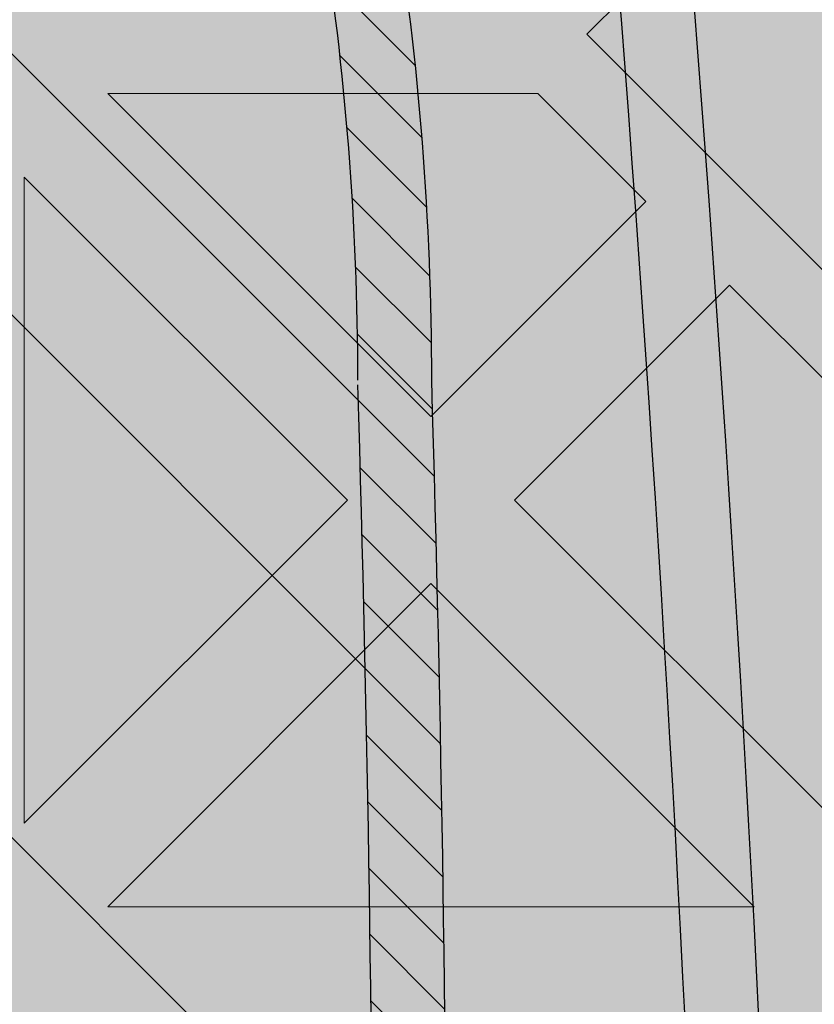
# Model space of a CAD drawing. Units: inches. Extents: x 844 to 2234, y 346 to 1084.
# Tile 38 of 93: x 1260.074 to 1261.788, y 699.229 to 701.353. Entities that reach past the tile are written whole.
import ezdxf

# ---------------------------------------------------------------- set-up
doc = ezdxf.new("R2010")
doc.units = ezdxf.units.IN
doc.header["$MEASUREMENT"] = 0
doc.layers.add('furniture', color=8, linetype='Continuous', lineweight=18)
doc.layers.add('RA-AP-01$0$INT', color=35, linetype='Continuous', lineweight=5)
doc.layers.add('RA-AP-01$0$FURN', color=3, linetype='Continuous')
doc.layers.add('RA-AP-01$0$WOOD', color=64, linetype='Continuous')

# ---------------------------------------------------------------- blocks, each defined once
blk = doc.blocks.new('A$C18D01794')
at = {"layer": 'RA-AP-01$0$INT'}
h = blk.add_hatch(color=256, dxfattribs=at)
h.paths.add_polyline_path([(4.585917135068448, -7.856712009587804), (4.614201406330596, -7.856712009587056), (4.668846067270487, -7.802067348644738), (4.723490728212344, -7.856712009584164), (4.771774999457151, -7.856712009582887), (4.826419660396886, -7.80206734864072), (4.862780050090322, -7.838427738332541), (4.844495778842715, -7.856712009580965), (4.862780050090411, -7.856712009580482), (4.905206456960182, -7.814285602707865), (4.947632863832445, -7.856712009578238), (4.965917135079675, -7.856712009577755), (4.947632863831759, -7.838427738330656), (4.983993253523576, -7.802067348637219), (5.038637914464627, -7.856712009575829), (5.08692218571208, -7.856712009574554), (5.141566846649976, -7.802067348634224), (5.196211507589851, -7.856712009571666), (5.224495778822615, -7.856712009570916), (4.905206456953975, -7.537422687702283)])
h.paths.add_polyline_path([(4.895206456956031, -7.575706958950402), (4.895206456958921, -7.684996280828174), (4.840561796018589, -7.630351619890275)], flags=16)
h.paths.add_polyline_path([(4.915206456955638, -7.575706958949956), (4.969851117895509, -7.630351619887399), (4.915206456957609, -7.684996280827732)], flags=16)
h.paths.add_polyline_path([(4.826419660395175, -7.644493755514321), (4.881064321335613, -7.699138416452331), (4.771774999456703, -7.69913841645522)], flags=16)
h.paths.add_polyline_path([(4.983993253519558, -7.644493755510815), (5.038637914460456, -7.699138416449285), (4.929348592581548, -7.69913841645126)], flags=16)
h.paths.add_polyline_path([(4.881064321336025, -7.719138416452334), (4.826419660397532, -7.773783077393256), (4.771774999457062, -7.719138416455217)], flags=16)
h.paths.add_polyline_path([(4.929348592582019, -7.71913841645126), (5.038637914460982, -7.719138416449284), (4.983993253522945, -7.773783077389749)], flags=16)
h.paths.add_polyline_path([(4.895206456960191, -7.733280552075633), (4.895206456962115, -7.806001331460164), (4.876922185715016, -7.824285602708492), (4.840561796021581, -7.787925213016675)], flags=16)
h.paths.add_polyline_path([(4.915206456958487, -7.733280552075187), (4.969851117899527, -7.787925213013798), (4.933490728206909, -7.824285602708034), (4.9152064569598, -7.806001331461736)], flags=16)
h.paths.add_polyline_path([(4.757632863832376, -7.733280552079264), (4.812277524772842, -7.787925213017304), (4.757632863834348, -7.842569873958233)], flags=16)
h.paths.add_polyline_path([(4.737632863832376, -7.73328055207979), (4.737632863834348, -7.842569873958701), (4.682988202893906, -7.787925213020692)], flags=16)
h.paths.add_polyline_path([(5.05278005008503, -7.733280552072701), (5.052780050087917, -7.842569873951664), (4.998135389146995, -7.787925213013169)], flags=16)
h.paths.add_polyline_path([(5.072780050085024, -7.733280552072333), (5.127424711025931, -7.787925213010806), (5.072780050087916, -7.842569873951244)], flags=16)
h.paths.add_polyline_path([(4.935917135072783, -7.506712009583784), (5.255206456948811, -7.826001331459767), (5.255206456948932, -7.797717060211899), (5.200561796010279, -7.743072399273238), (5.255206456949403, -7.688427738334128), (5.25520645694961, -7.640143467086677), (5.200561796009787, -7.585498806146837), (5.236922185702417, -7.549138416454212), (5.255206456949919, -7.56742268770172), (5.255206456949998, -7.549138416454178), (5.212780050078687, -7.506712009583814), (5.25520645695036, -7.464285602712145), (5.255206456950438, -7.446001331464763), (5.236922185702424, -7.464285602712779), (5.200561796009796, -7.427925213020149), (5.255206456950753, -7.373280552079203), (5.25520645695096, -7.324996280834394), (5.200561796010322, -7.270351619893748), (5.255206456951428, -7.215706958952649), (5.255206456951547, -7.187422687705071)])
h.paths.add_polyline_path([(5.042988202883395, -7.42792521302065), (5.097632863823085, -7.373280552080975), (5.097632863822622, -7.482569873959883)], flags=16)
h.paths.add_polyline_path([(5.028846067259663, -7.442067348644384), (5.083490728198774, -7.496712009583504), (4.974201406321001, -7.496712009583035)], flags=16)
h.paths.add_polyline_path([(5.117632863823087, -7.37328055208089), (5.172277524762331, -7.42792521302015), (5.11763286382262, -7.482569873959851)], flags=16)
h.paths.add_polyline_path([(5.08349072819877, -7.516712009582191), (5.028846067259652, -7.571356670521302), (4.974201406320998, -7.516712009582638)], flags=16)
h.paths.add_polyline_path([(5.131774999446817, -7.35913841645716), (5.186419660386065, -7.413783077396415), (5.241064321325782, -7.359138416456712)], flags=17)
h.paths.add_polyline_path([(5.131774999446228, -7.496712009583703), (5.186419660386065, -7.442067348643883), (5.222780050079488, -7.478427738337313), (5.204495778832781, -7.496712009584014)], flags=16)
h.paths.add_polyline_path([(5.097632863822613, -7.530854145205813), (5.097632863823061, -7.640143467084723), (5.042988202883383, -7.585498806145032)], flags=16)
h.paths.add_polyline_path([(5.131774999446899, -7.339138416457162), (5.241064321325809, -7.339138416456712), (5.186419660386591, -7.284493755517479)], flags=17)
h.paths.add_polyline_path([(5.131774999446226, -7.516712009581999), (5.204495778830767, -7.516712009581702), (5.22278005007868, -7.534996280829206), (5.186419660386049, -7.571356670521828)], flags=16)
h.paths.add_polyline_path([(5.11763286382262, -7.530854145205852), (5.17227752476232, -7.585498806145562), (5.117632863823064, -7.64014346708481)], flags=16)
h.paths.add_polyline_path([(5.186419660386069, -7.599640941770585), (5.241064321325754, -7.654285602710281), (5.131774999446791, -7.654285602709814)], flags=16)
h.paths.add_polyline_path([(5.131774999446872, -7.674285602709813), (5.24106432132578, -7.674285602710282), (5.186419660386554, -7.728930263649504)], flags=16)
h.paths.add_polyline_path([(5.255206456951811, -7.126001331467467), (5.255206456951895, -7.106712009588038), (4.555206456956052, -7.106712009588038), (4.555206456956136, -7.12600133146746), (4.905206456953973, -7.476001331465289)])
h.paths.add_polyline_path([(4.983993253513404, -7.368930263651977), (4.92934859257295, -7.314285602713969), (5.03863791445186, -7.314285602711063)], flags=16)
h.paths.add_polyline_path([(4.969851117889988, -7.383072399276016), (4.915206456952556, -7.437717060215906), (4.915206456949648, -7.328427738338133)], flags=16)
h.paths.add_polyline_path([(4.929348592572535, -7.294285602713971), (4.983993253511019, -7.239640941773039), (5.038637914451496, -7.294285602711065)], flags=16)
h.paths.add_polyline_path([(5.052780050074912, -7.280143467087016), (4.998135389134438, -7.225498806148989), (5.052780050072919, -7.170854145208052)], flags=16)
h.paths.add_polyline_path([(5.07278005007491, -7.280143467086489), (5.072780050072918, -7.170854145207579), (5.127424711013374, -7.225498806145578)], flags=16)
h.paths.add_polyline_path([(4.89520645695295, -7.437717060216355), (4.840561796013067, -7.383072399278919), (4.895206456950961, -7.328427738338582)], flags=16)
h.paths.add_polyline_path([(4.915206456948365, -7.280143467090674), (4.915206456946434, -7.207422687704125), (4.933490728192729, -7.18913841645701), (4.969851117886972, -7.225498806149623)], flags=16)
h.paths.add_polyline_path([(4.881064321327021, -7.314285602715054), (4.82641966038902, -7.368930263655506), (4.771774999448108, -7.314285602717047)], flags=16)
h.paths.add_polyline_path([(4.895206456950073, -7.280143467091125), (4.840561796009022, -7.225498806152518), (4.876922185700835, -7.18913841645908), (4.895206456948749, -7.207422687706589)], flags=16)
h.paths.add_polyline_path([(4.983993253510392, -7.211356670525576), (4.947632863816944, -7.174996280833758), (4.965917135064043, -7.156712009585847), (5.038637914448995, -7.156712009584522)], flags=16)
h.paths.add_polyline_path([(4.881064321326543, -7.294285602715056), (4.771774999447578, -7.294285602717046), (4.826419660385607, -7.239640941776569)], flags=16)
h.paths.add_polyline_path([(4.905206456946447, -7.19913841645844), (4.862780050074785, -7.156712009587725), (4.947632863816685, -7.156712009586302)], flags=16)
h.paths.add_polyline_path([(5.14156684663679, -7.211356670521528), (5.086922185696452, -7.156712009583639), (5.196211507574223, -7.156712009581651)], flags=16)
h.paths.add_polyline_path([(4.8264196603837, -7.211356670529104), (4.771774999442643, -7.156712009590501), (4.8444957788276, -7.156712009588568), (4.862780050075511, -7.17499628083566)], flags=16)
h.paths.add_polyline_path([(4.812277524760289, -7.225498806153156), (4.757632863822258, -7.28014346709363), (4.757632863819352, -7.170854145214669)], flags=16)
h.paths.add_polyline_path([(4.73763286382226, -7.280143467093997), (4.682988202881349, -7.22549880615554), (4.737632863819352, -7.170854145215086)], flags=16)
h.paths.add_polyline_path([(4.723490728195188, -7.156712009591787), (4.668846067257299, -7.211356670532127), (4.614201406317417, -7.156712009594693)], flags=16)
h.paths.add_polyline_path([(4.597632863829262, -7.506712009583814), (4.555206456957951, -7.54913841645418), (4.555206456958029, -7.56742268770172), (4.573490728205535, -7.549138416454212), (4.609851117898167, -7.585498806146839), (4.555206456958338, -7.640143467086675), (4.555206456958546, -7.688427738334125), (4.60985111789767, -7.743072399273238), (4.555206456959015, -7.797717060211899), (4.555206456959138, -7.826001331459767), (4.874495778835167, -7.506712009583786), (4.5552064569564, -7.187422687705062), (4.555206456956523, -7.215706958952644), (4.609851117897629, -7.270351619893746), (4.555206456956988, -7.324996280834396), (4.555206456957198, -7.373280552079195), (4.609851117898153, -7.427925213020147), (4.573490728205528, -7.464285602712779), (4.555206456957507, -7.446001331464756), (4.555206456957585, -7.464285602712143)])
h.paths.add_polyline_path([(4.712780050085332, -7.482569873959882), (4.712780050084863, -7.373280552080972), (4.767424711024555, -7.42792521302065)], flags=16)
h.paths.add_polyline_path([(4.726922185709173, -7.496712009583504), (4.781566846648288, -7.442067348644384), (4.836211507586949, -7.496712009583033)], flags=16)
h.paths.add_polyline_path([(4.692780050085327, -7.482569873959851), (4.638135389145619, -7.427925213020149), (4.692780050084865, -7.373280552080892)], flags=16)
h.paths.add_polyline_path([(4.726922185709182, -7.516712009582191), (4.836211507586949, -7.51671200958264), (4.7815668466483, -7.571356670521304)], flags=16)
h.paths.add_polyline_path([(4.678637914461726, -7.496712009583706), (4.605917135075169, -7.496712009584014), (4.587632863828464, -7.478427738337311), (4.623993253521887, -7.442067348643881)], flags=16)
h.paths.add_polyline_path([(4.712780050085336, -7.530854145205816), (4.767424711024568, -7.585498806145034), (4.71278005008489, -7.640143467084724)], flags=16)
h.paths.add_polyline_path([(4.678637914461726, -7.516712009582001), (4.623993253521899, -7.571356670521829), (4.587632863829271, -7.534996280829206), (4.605917135077185, -7.5167120095817)], flags=16)
h.paths.add_polyline_path([(4.692780050085336, -7.530854145205848), (4.692780050084889, -7.64014346708481), (4.638135389145632, -7.585498806145562)], flags=16)
h.paths.add_polyline_path([(4.623993253521885, -7.413783077396415), (4.678637914461131, -7.359138416457161), (4.56934859258217, -7.359138416456712)], flags=17)
h.paths.add_polyline_path([(4.623993253521901, -7.599640941770568), (4.678637914461158, -7.654285602709814), (4.569348592582195, -7.654285602710281)], flags=16)
h.paths.add_polyline_path([(4.678637914461051, -7.339138416457162), (4.623993253521361, -7.284493755517479), (4.569348592582143, -7.339138416456712)], flags=17)
h.paths.add_polyline_path([(4.678637914461076, -7.674285602709813), (4.623993253521399, -7.728930263649504), (4.569348592582167, -7.674285602710281)], flags=16)
h = blk.add_hatch(color=256, dxfattribs=at)
h.paths.add_polyline_path([(4.781566846647504, -7.442067348645805), (4.836211507586161, -7.496712009584463), (4.726922185708388, -7.496712009584918)])
h.paths.add_polyline_path([(4.836211507586161, -7.516712009584068), (4.781566846647504, -7.571356670522723), (4.726922185708388, -7.516712009583606)])
h.paths.add_polyline_path([(4.76742471102377, -7.585498806146453), (4.712780050084083, -7.640143467086137), (4.712780050084542, -7.530854145207227)])
h.paths.add_polyline_path([(4.692780050084544, -7.530854145207257), (4.692780050084084, -7.64014346708622), (4.638135389144834, -7.585498806146965)])
h.paths.add_polyline_path([(4.678637914460932, -7.516712009583407), (4.623993253521102, -7.571356670523233), (4.587632863827676, -7.53499628082981), (4.605917135074382, -7.516712009583104)])
h.paths.add_polyline_path([(4.573490728204743, -7.54913841645434), (4.60985111789737, -7.585498806146969), (4.555206456957541, -7.640143467086797), (4.555206456957237, -7.567422687701846)])
h.paths.add_polyline_path([(4.623993253521098, -7.599640941770699), (4.67863791446035, -7.654285602709951), (4.56934859258139, -7.654285602710407)])
h.paths.add_polyline_path([(4.678637914460275, -7.67428560270995), (4.623993253520583, -7.728930263649637), (4.56934859258136, -7.674285602710405)])
h.paths.add_polyline_path([(4.609851117896854, -7.743072399273369), (4.555206456958196, -7.797717060212026), (4.555206456957738, -7.688427738334254)])
h.paths.add_polyline_path([(4.597632863828475, -7.506712009583301), (4.555206456957283, -7.549138416454495), (4.555206456956805, -7.464285602712587)])
h.paths.add_polyline_path([(4.678637914460932, -7.496712009585113), (4.605917135076396, -7.496712009585417), (4.587632863828479, -7.478427738337913), (4.623993253521104, -7.442067348645284)])
h.paths.add_polyline_path([(4.692780050084091, -7.373280552082301), (4.692780050084548, -7.482569873961267), (4.638135389144834, -7.427925213021552)])
h.paths.add_polyline_path([(4.767424711023772, -7.427925213022072), (4.712780050084545, -7.48256987396129), (4.712780050084089, -7.373280552082384)])
h.paths.add_polyline_path([(4.67863791446036, -7.359138416457298), (4.623993253521105, -7.41378307739655), (4.569348592581399, -7.35913841645684)])
h.paths.add_polyline_path([(4.609851117897371, -7.427925213020278), (4.573490728204743, -7.464285602712907), (4.555206456957237, -7.446001331465401), (4.555206456957548, -7.373280552080448)])
h.paths.add_polyline_path([(4.623993253520596, -7.284493755517612), (4.67863791446028, -7.339138416457299), (4.569348592581367, -7.339138416456838)])
h.paths.add_polyline_path([(4.609851117896867, -7.270351619893878), (4.555206456957749, -7.324996280832994), (4.55520645695821, -7.21570695895522)])
for p, q in [((4.678637914461133, -7.359138416457161), (4.56934859258217, -7.359138416456712)), ((4.56934859258217, -7.359138416456712), (4.623993253521885, -7.413783077396415)), ((4.678637914461133, -7.359138416457161), (4.623993253521885, -7.413783077396415)), ((4.555206456958322, -7.373280552080322), (4.609851117898155, -7.427925213020149)), ((4.692780050084865, -7.37328055208089), (4.638135389145619, -7.427925213020149)), ((4.692780050084865, -7.37328055208089), (4.692780050085331, -7.482569873959853)), ((4.609851117898155, -7.427925213020147), (4.573490728205528, -7.464285602712779)), ((4.692780050085331, -7.482569873959853), (4.638135389145619, -7.427925213020149)), ((4.623993253521889, -7.442067348643881), (4.587632863829264, -7.478427738336511)), ((4.678637914461721, -7.496712009583704), (4.623993253521887, -7.442067348643881)), ((4.555206456958022, -7.446001331465273), (4.573490728205528, -7.464285602712781)), ((4.573490728205528, -7.464285602712779), (4.55520645695807, -7.446001331465319)), ((4.597632863829264, -7.506712009583814), (4.55520645695807, -7.464285602712626)), ((4.605917135075176, -7.496712009584021), (4.587632863827669, -7.478427738336517)), ((4.60591713507677, -7.496712009584014), (4.678637914461721, -7.496712009583704)), ((4.597632863829264, -7.506712009583814), (4.555206456957598, -7.549138416454534))]:
    blk.add_line(p, q, dxfattribs=at)
blk = doc.blocks.new('A$C32926AE1')
at = {"layer": 'RA-AP-01$0$WOOD'}
h = blk.add_hatch(color=256, dxfattribs=at)
h.dxf.hatch_style = 1
h.paths.add_polyline_path([(5.157430609644524, 4.573483066760929, -0.1009492694046607), (5.155401577623758, 4.593365984175333, -0.1842662638101597), (5.172249623284174, 4.638795604568598, 0.2056608120311276), (5.179560981299304, 4.661316324430096, 0.3614336704623542), (5.134352340494423, 4.706524965234944, 0.2056608120311297), (5.111831620632933, 4.699213607219793, -0.1842662638101113), (5.066402000239693, 4.682365561559342, -0.1055311479399994), (5.045656153913092, 4.68467289944697, 0.1567636581983829), (4.763886414745334, 4.684672899446966, -0.1055311479399895), (4.743140568418733, 4.68236556155934, -0.1842662638100833), (4.6977109480255, 4.69921360721979, 0.2056608120302612), (4.675190228164109, 4.706524965234949, 0.3614336704708441), (4.629981587358889, 4.66131632442871, 0.2056608120245944), (4.637292945374126, 4.638795604567974, -0.1842662638101024), (4.654140991034615, 4.59336598417475, -0.1009492694055169), (4.652111959013835, 4.573483066760181, 0.021410119221476), (4.629748025606143, 4.156712009541676, 0.0214101192214795), (4.652111959013809, 3.739940952323101, -0.1009492694059586), (4.654140991034615, 3.720058034908448, -0.1842662638100975), (4.637292945374126, 3.674628414515226, 0.2056608120245705), (4.629981587358889, 3.652107694654492, 0.3614336704708879), (4.675190228164113, 3.606899053848249, 0.2056608120302384), (4.697710948025501, 3.614210411863408, -0.1842662638100995), (4.743140568418738, 3.63105845752386, -0.1055311479402541), (4.763886414745388, 3.628751119636215, 0.1567636581983776), (5.045656153913137, 3.628751119636244, -0.1055311479397538), (5.066402000239692, 3.631058457523857, -0.1842662638101067), (5.111831620632931, 3.614210411863407, 0.2056608120310924), (5.134352340494417, 3.606899053848256, 0.3614336704624001), (5.179560981299307, 3.652107694653103, 0.2056608120311314), (5.172249623284175, 3.6746284145146, -0.1842662638101402), (5.155401577623758, 3.72005803490786, -0.1009492694051366), (5.15743060964455, 3.739940952322354, 0.0214101192215073), (5.179794543052287, 4.156712009541468, 0.0214101192215252)])
h.paths.add_polyline_path([(4.639748609479751, 4.156712009541513, 0.0213537860821624), (4.661970494867118, 3.741887061152232, -0.094075836301374), (4.664143710413708, 3.7196126951003, -0.1824818158568985), (4.644813765429836, 3.668037719127816, 0.2056608120245319), (4.639939526753007, 3.653023905887301, 0.3614336704710246), (4.676106439397173, 3.616856993242342, 0.2056608120302234), (4.691120252638095, 3.621731231919122, -0.1824818158602558), (4.742695228611606, 3.641061176902986, -0.1029891339458722), (4.766991894714349, 3.638256818950944, 0.156709409989566), (5.042550673941472, 3.638256818950105, -0.102989133958497), (5.066847340047078, 3.641061176902949, -0.1824818158594995), (5.118422316020358, 3.621731231919103, 0.2056608120311416), (5.133436129261316, 3.616856993242346, 0.3614336704621468), (5.169603041905217, 3.653023905886178, 0.2056608120310986), (5.164728803228477, 3.668037719127177, -0.1824818158565612), (5.145398858244737, 3.719612695099578, -0.0940758363009313), (5.147572073791232, 3.741887061151398, 0.0213537860822023), (5.169793959178681, 4.156712009541451, 0.0213537860822226), (5.147572073791203, 4.571536957931898, -0.0940758363005034), (5.145398858244737, 4.59381132398362, -0.1824818158565587), (5.164728803228476, 4.645386299956021, 0.2056608120311045), (5.169603041905216, 4.66040011319702, 0.3614336704621845), (5.133436129261313, 4.696567025840856, 0.2056608120310773), (5.118422316020359, 4.691692787164098, -0.182481815859508), (5.066847340047078, 4.67236284218025, -0.1029891339584606), (5.04255067394148, 4.675167200133092, 0.156709409989566), (4.766991894714357, 4.675167200132257, -0.1029891339458842), (4.742695228611611, 4.672362842180213, -0.1824818158602725), (4.691120252638095, 4.691692787164077, 0.2056608120302152), (4.676106439397174, 4.696567025840858, 0.3614336704710363), (4.639939526753005, 4.660400113195899, 0.2056608120245495), (4.644813765429837, 4.645386299955384, -0.1824818158568934), (4.664143710413708, 4.593811323982902, -0.0940758363009187), (4.661970494867149, 4.571536957931074, 0.021353786082177)], flags=16)
h.paths.add_polyline_path([(5.129794543052235, 4.432167055276933, -0.0141661062790638), (5.130152669293814, 4.156927903047693, -0.0141661062790647), (5.129794543052234, 3.881688750818433, -0.0785247771143638), (5.10979738006795, 3.755143611847103, 0.0945969212073497), (5.105408519571111, 3.717898134952927, 0.1043170707844957), (5.116074640131521, 3.670385395016088, 0.1043170707864965), (5.068561900193738, 3.681051515576561, 0.09459692119553), (5.031316423304057, 3.676662655080835, -0.1580239521427272), (4.778226145355827, 3.676662655080367, 0.0945969211986668), (4.740980668464973, 3.681051515576592, 0.1043170707882822), (4.693467928526415, 3.670385395015844, 0.1043170707867916), (4.704134049087309, 3.717898134953662, 0.0945969211972894), (4.69974518859162, 3.755143611844042, -0.0785247771163196), (4.679748025606343, 3.881688750818406, -0.0141661062790663), (4.679389899364763, 4.156927903047693, -0.0141661062790672), (4.679748025606343, 4.432167055276998, -0.0785247771163064), (4.699745188591625, 4.55871219425134, 0.094596921197333), (4.704134049087308, 4.595957671141738, 0.1043170707867205), (4.693467928526416, 4.643470411079523, 0.1043170707882628), (4.740980668464965, 4.632804290518776, 0.0945969211988114), (4.778226145355874, 4.637193151015016, -0.158023952142669), (5.031316423304015, 4.637193151014546, 0.0945969211956361), (5.068561900193736, 4.632804290518806, 0.1043170707864979), (5.11607464013152, 4.643470411079278, 0.1043170707844617), (5.105408519571112, 4.595957671142455, 0.0945969212074597), (5.109797380067959, 4.558712194248236, -0.0785247771143467)], flags=0)
h.paths.add_polyline_path([(5.119794532311105, 4.432259799204851, -0.0142000800617244), (5.120156169157484, 4.156927903047701, -0.0142000800617277), (5.119794532311105, 3.881596006890482, -0.0784894509520253), (5.100273383573699, 3.758192358677797, 0.0940138827242913), (5.095413455884425, 3.717477693979438, 0.0606271852308753), (5.099615656341024, 3.686844378806616, 0.0606271852322524), (5.068982341167493, 3.691046579263239, 0.0940138827010453), (5.028267676478798, 3.686186651576848, -0.1580706864508061), (4.781274892180912, 3.686186651576435, 0.0940138827026903), (4.740560227491556, 3.691046579263279, 0.0606271852339895), (4.709926912317155, 3.686844378806508, 0.0606271852329405), (4.714129112773991, 3.717477693980356, 0.094013882701304), (4.709269185087677, 3.758192358669163, -0.0784894509577193), (4.689748036347473, 3.881596006890469, -0.014200080061729), (4.689386399501094, 4.156927903047709, -0.0142000800617217), (4.689748036347473, 4.432259799204808, -0.078489450957724), (4.709269185087651, 4.555663447426125, 0.0940138827014585), (4.714129112773992, 4.596378112114996, 0.0606271852329731), (4.709926912317154, 4.62701142728886, 0.0606271852340196), (4.74056022749157, 4.622809226832087, 0.0940138827024997), (4.781274892180847, 4.627669154518912, -0.1580706864508359), (5.028267676478777, 4.627669154518526, 0.0940138827010946), (5.068982341167492, 4.622809226832129, 0.060627185232254), (5.099615656341024, 4.627011427288751, 0.0606271852308727), (5.095413455884425, 4.59637811211593, 0.0940138827241088), (5.100273383573675, 4.555663447417647, -0.0784894509520978)], flags=0)
h.paths.add_polyline_path([(5.06978912287499, 4.430218106756144, -0.014241683694547), (5.070173729147532, 4.156927903047672, -0.0142416836945458), (5.06978912287499, 3.883637699339223, -0.0800609523125196), (5.052662118612511, 3.773463122773442, 0.0526421978001116), (5.04590916754064, 3.740550867606997, 0.0526421977992423), (5.012996912374707, 3.73379791653534, -0.1583028414718258), (4.796545656286308, 3.73379791653451, 0.0526421978034211), (4.763633401117837, 3.740550867607021, 0.0526421978018622), (4.756880450045755, 3.773463122774558, -0.0800609523117106), (4.739753445783639, 3.883637699339268, -0.0142416836945435), (4.739368839511098, 4.156927903047671, -0.0142416836945477), (4.739753445783639, 4.430218106756155, -0.0800609523116345), (4.75688045004574, 4.540392683320762, 0.052642197801941), (4.763633401117837, 4.573304938488346, 0.0526421978035071), (4.796545656286361, 4.580057889560873, -0.1583028414717561), (5.012996912374669, 4.580057889560039, 0.0526421977993048), (5.04590916754064, 4.57330493848837, 0.0526421978002057), (5.052662118612529, 4.540392683321868, -0.080060952312477)], flags=0)
h.paths.add_polyline_path([(5.049789715110557, 4.43038092723357, -0.0143097550741839), (5.05018085590259, 4.156927903047715, -0.0143097550741854), (5.049789715110558, 3.883474878861827, -0.0800685599149176), (5.03362098255317, 3.779581877367999, 0.0306258898956367), (5.028241146483733, 3.758218888663947, 0.0306258898977031), (5.006878157778253, 3.75283905259408, -0.1583983521624096), (4.802664410878162, 3.752839052594731, 0.0306258898946014), (4.781301422174808, 3.758218888663924, 0.0306258898967912), (4.775921586105202, 3.779581877368794, -0.080068559914251), (4.759752853548071, 3.883474878861786, -0.0143097550741854), (4.759361712756037, 4.156927903047671, -0.0143097550741854), (4.759752853548071, 4.430380927233557, -0.0800685599142479), (4.775921586105193, 4.534273928726546, 0.0306258898968306), (4.781301422174808, 4.555636917431444, 0.0306258898945754), (4.802664410878143, 4.561016753500631, -0.1583983521624168), (5.006878157778244, 4.561016753501291, 0.0306258898977177), (5.028241146483733, 4.555636917431421, 0.0306258898958182), (5.03362098255321, 4.534273928727244, -0.080068559914796)], flags=0)
h.paths.add_polyline_path([(4.999766070382627, 4.428171244713864, -0.0143443147609634), (5.000198441819402, 4.156927903047689, -0.0143443147609612), (4.999766070382627, 3.885684561381556, -0.0784641635803329), (4.987356730658798, 3.799103304488872, -0.1506053783831347), (4.822185837999821, 3.79910330448882, -0.0784641635803318), (4.809776498276007, 3.885684561381509, -0.014344314760963), (4.809344126839227, 4.156927903047677, -0.0143443147609645), (4.809776498276007, 4.428171244713873, -0.0784641635803192), (4.822185837999822, 4.514752501606549, -0.1506053783831338), (4.987356730658798, 4.514752501606494, -0.078464163580285)], flags=0)
h.paths.add_polyline_path([(4.979755254238824, 4.42764379880488, -0.0143772539198268), (4.980205517789977, 4.156927903047693, -0.0143772539198275), (4.979755254238824, 3.886212007290489, -0.0689242507424422), (4.971183264704897, 3.815276770442801, -0.1296645318904179), (4.838359303953726, 3.815276770442746, -0.0689242507424186), (4.829787314419809, 3.886212007290419, -0.0143772539198292), (4.829337050868653, 4.156927903047653, -0.0143772539198325), (4.829787314419809, 4.427643798804946, -0.0689242507424211), (4.838359303953725, 4.498579035652621, -0.1296645318904187), (4.971183264704897, 4.498579035652565, -0.0689242507424401)], flags=0)
h = blk.add_hatch(color=256, dxfattribs=at)
h.dxf.hatch_style = 1
h.paths.add_polyline_path([(5.145398858244737, 4.59381132398362, -0.1824818158565616), (5.164728803228476, 4.645386299956021, 0.2056608120311045), (5.169603041905216, 4.66040011319702, 0.3614336704621845), (5.133436129261313, 4.696567025840856, 0.2056608120310773), (5.118422316020359, 4.691692787164098, -0.182481815859508), (5.066847340047078, 4.67236284218025, -0.1029891339584606), (5.04255067394148, 4.675167200133092, 0.156709409989566), (4.766991894714357, 4.675167200132257, -0.1029891339458842), (4.742695228611611, 4.672362842180213, -0.1824818158602725), (4.691120252638095, 4.691692787164077, 0.2056608120302152), (4.676106439397174, 4.696567025840858, 0.3614336704710363), (4.639939526753005, 4.660400113195899, 0.2056608120245495), (4.644813765429837, 4.645386299955384, -0.1824818158568934), (4.664143710413708, 4.593811323982902, -0.0940758363009187), (4.661970494867149, 4.571536957931074, 0.0213537860821772), (4.639748609479751, 4.156712009541507, 0.0213537860821625), (4.661970494867119, 3.741887061152226, -0.0940758363013071), (4.664143710413708, 3.719612695100309, -0.1824818158569294), (4.644813765429836, 3.668037719127816, 0.2056608120245319), (4.639939526753007, 3.653023905887301, 0.3614336704710246), (4.676106439397173, 3.616856993242342, 0.2056608120302234), (4.691120252638095, 3.621731231919122, -0.1824818158602558), (4.742695228611606, 3.641061176902986, -0.1029891339458722), (4.766991894714349, 3.638256818950944, 0.156709409989566), (5.042550673941472, 3.638256818950105, -0.102989133958497), (5.066847340047078, 3.641061176902949, -0.1824818158594995), (5.118422316020358, 3.621731231919103, 0.2056608120311416), (5.133436129261316, 3.616856993242346, 0.3614336704621468), (5.169603041905217, 3.653023905886178, 0.2056608120310986), (5.164728803228477, 3.668037719127177, -0.1824818158565612), (5.145398858244737, 3.719612695099578, -0.0940758363009313), (5.147572073791232, 3.741887061151398, 0.0213537860822023), (5.169793959178681, 4.156712009541451, 0.0213537860822226), (5.147572073791203, 4.571536957931898, -0.0940758363004996)])
h.paths.add_polyline_path([(5.109797380067958, 4.55871219424824, -0.0785247771143472), (5.129794543052234, 4.432167055276936, -0.0141661062790644), (5.130152669293814, 4.156927903047685, -0.014166106279066), (5.129794543052234, 3.881688750818401, -0.0785247771143517), (5.109797380067946, 3.755143611847092, 0.0945969212073132), (5.105408519571111, 3.717898134952929, 0.1043170707844995), (5.116074640131521, 3.670385395016088, 0.1043170707864965), (5.068561900193738, 3.681051515576561, 0.09459692119553), (5.031316423304057, 3.676662655080835, -0.1580239521427272), (4.778226145355827, 3.676662655080367, 0.0945969211986668), (4.740980668464973, 3.681051515576592, 0.1043170707882822), (4.693467928526415, 3.670385395015844, 0.1043170707867916), (4.704134049087309, 3.717898134953662, 0.0945969211972894), (4.69974518859162, 3.755143611844042, -0.0785247771163196), (4.679748025606343, 3.881688750818406, -0.0141661062790663), (4.679389899364763, 4.156927903047693, -0.0141661062790672), (4.679748025606343, 4.432167055276998, -0.0785247771163064), (4.699745188591625, 4.55871219425134, 0.094596921197333), (4.704134049087308, 4.595957671141738, 0.1043170707867205), (4.693467928526416, 4.643470411079523, 0.1043170707882628), (4.740980668464965, 4.632804290518776, 0.0945969211988114), (4.778226145355874, 4.637193151015016, -0.158023952142669), (5.031316423304015, 4.637193151014546, 0.0945969211956361), (5.068561900193736, 4.632804290518806, 0.1043170707864979), (5.11607464013152, 4.643470411079278, 0.1043170707844617), (5.105408519571112, 4.595957671142455, 0.0945969212074504)], flags=16)
h.paths.add_polyline_path([(5.100273383573655, 4.55566344741771, -0.0784894509521388), (5.119794532311105, 4.432259799204852, -0.0142000800617252), (5.120156169157484, 4.156927903047686, -0.014200080061726), (5.119794532311105, 3.881596006890502, -0.0784894509520446), (5.100273383573696, 3.758192358677786, 0.0940138827242721), (5.095413455884425, 3.717477693979436, 0.0606271852308692), (5.099615656341024, 3.686844378806616, 0.0606271852322522), (5.068982341167493, 3.691046579263239, 0.0940138827010453), (5.028267676478798, 3.686186651576848, -0.1580706864508061), (4.781274892180912, 3.686186651576435, 0.0940138827026903), (4.740560227491556, 3.691046579263279, 0.0606271852339895), (4.709926912317155, 3.686844378806508, 0.0606271852329405), (4.714129112773991, 3.717477693980356, 0.094013882701304), (4.709269185087677, 3.758192358669163, -0.0784894509577193), (4.689748036347473, 3.881596006890469, -0.014200080061729), (4.689386399501094, 4.156927903047709, -0.0142000800617217), (4.689748036347473, 4.432259799204808, -0.078489450957724), (4.709269185087651, 4.555663447426125, 0.0940138827014585), (4.714129112773992, 4.596378112114996, 0.0606271852329731), (4.709926912317154, 4.62701142728886, 0.0606271852340196), (4.74056022749157, 4.622809226832087, 0.0940138827024997), (4.781274892180847, 4.627669154518912, -0.1580706864508359), (5.028267676478777, 4.627669154518526, 0.0940138827010946), (5.068982341167492, 4.622809226832129, 0.060627185232254), (5.099615656341024, 4.627011427288751, 0.0606271852308727), (5.095413455884425, 4.59637811211593, 0.094013882723957)], flags=0)
h.paths.add_polyline_path([(5.04590916754064, 4.57330493848837, 0.0526421978002057), (5.052662118612529, 4.540392683321868, -0.0800609523124783), (5.06978912287499, 4.430218106756142, -0.0142416836945469), (5.070173729147532, 4.156927903047672, -0.0142416836945458), (5.06978912287499, 3.883637699339223, -0.0800609523125196), (5.052662118612511, 3.773463122773442, 0.0526421978001116), (5.04590916754064, 3.740550867606997, 0.0526421977992423), (5.012996912374707, 3.73379791653534, -0.1583028414718258), (4.796545656286308, 3.73379791653451, 0.0526421978034211), (4.763633401117837, 3.740550867607021, 0.0526421978018622), (4.756880450045755, 3.773463122774558, -0.0800609523117106), (4.739753445783639, 3.883637699339268, -0.0142416836945435), (4.739368839511098, 4.156927903047671, -0.0142416836945477), (4.739753445783639, 4.430218106756155, -0.0800609523116345), (4.75688045004574, 4.540392683320762, 0.052642197801941), (4.763633401117837, 4.573304938488346, 0.0526421978035071), (4.796545656286361, 4.580057889560873, -0.1583028414717561), (5.012996912374669, 4.580057889560039, 0.0526421977993048)], flags=0)
h.paths.add_polyline_path([(5.028241146483733, 4.555636917431422, 0.0306258898956949), (5.033620982553182, 4.534273928727329, -0.0800685599148649), (5.049789715110557, 4.430380927233569, -0.0143097550741839), (5.05018085590259, 4.156927903047715, -0.0143097550741854), (5.049789715110558, 3.883474878861827, -0.0800685599149176), (5.03362098255317, 3.779581877367999, 0.0306258898956367), (5.028241146483733, 3.758218888663947, 0.0306258898977031), (5.006878157778253, 3.75283905259408, -0.1583983521624096), (4.802664410878162, 3.752839052594731, 0.0306258898946014), (4.781301422174808, 3.758218888663924, 0.0306258898967912), (4.775921586105202, 3.779581877368794, -0.080068559914251), (4.759752853548071, 3.883474878861786, -0.0143097550741854), (4.759361712756037, 4.156927903047671, -0.0143097550741854), (4.759752853548071, 4.430380927233557, -0.0800685599142479), (4.775921586105193, 4.534273928726546, 0.0306258898968306), (4.781301422174808, 4.555636917431444, 0.0306258898945754), (4.802664410878143, 4.561016753500631, -0.1583983521624168), (5.006878157778244, 4.561016753501291, 0.0306258898977174)], flags=0)
h.paths.add_polyline_path([(4.987356730658798, 4.514752501606494, -0.0784641635803018), (4.999766070382627, 4.428171244713845, -0.0143443147609637), (5.000198441819402, 4.156927903047665, -0.0143443147609622), (4.999766070382628, 3.885684561381514, -0.0784641635802952), (4.987356730658797, 3.799103304488872, -0.1506053783831338), (4.822185837999821, 3.799103304488819, -0.0784641635803342), (4.809776498276007, 3.885684561381512, -0.0143443147609628), (4.809344126839227, 4.156927903047676, -0.0143443147609646), (4.809776498276007, 4.428171244713873, -0.0784641635803192), (4.822185837999822, 4.514752501606549, -0.1506053783831338)], flags=0)
h.paths.add_polyline_path([(4.971183264704897, 4.498579035652566, -0.0689242507424384), (4.979755254238824, 4.427643798804883, -0.0143772539198276), (4.980205517789977, 4.15692790304768, -0.0143772539198258), (4.979755254238823, 3.88621200729051, -0.0689242507424628), (4.971183264704897, 3.815276770442801, -0.129664531890417), (4.838359303953726, 3.815276770442746, -0.0689242507424186), (4.829787314419809, 3.886212007290419, -0.0143772539198292), (4.829337050868653, 4.156927903047653, -0.0143772539198325), (4.829787314419809, 4.427643798804946, -0.0689242507424211), (4.838359303953725, 4.498579035652621, -0.1296645318904187)], flags=0)
h = blk.add_hatch(dxfattribs=at)
h.set_pattern_fill('ANSI31', color=256, scale=0.05, style=0)
h.set_pattern_definition([(45, (0, 0), (-0.0044194173824159, 0.0044194173824159), [])])
h.paths.add_polyline_path([(5.130152669293814, 4.156927903047704, 0.0141661062790657), (5.129794543052234, 4.432167055276982, 0.0777827904001433), (5.110168979996553, 4.557559993161921, -0.0976515123401879), (5.105408519571111, 4.595957671142454, -0.1043170707844687), (5.116074640131522, 4.64347041107928), (5.099615656341024, 4.627011427288751, 0.0606271852308727), (5.095413455884425, 4.59637811211593, 0.0940138827241088), (5.100273383573675, 4.555663447417647, -0.0784894509520972), (5.119794532311105, 4.432259799204852, -0.0142000800617252), (5.120156169157484, 4.156927903047686, -0.014200080061726), (5.119794532311105, 3.881596006890502, -0.0784894509520446), (5.100273383573696, 3.758192358677786, 0.0940138827242721), (5.095413455884425, 3.717477693979436, 0.0606271852308692), (5.099615656341024, 3.686844378806616), (5.116074640131519, 3.67038539501609, -0.1043170707844594), (5.105408519571112, 3.717898134952912, -0.0976515123401594), (5.11016897999655, 3.756295812933435, 0.0777827904001654), (5.129794543052234, 3.881688750818409, 0.0141661062790665)])
h.paths.add_polyline_path([(5.030164222210597, 3.676291055149937, -0.0976515123472002), (5.068561900193739, 3.681051515576561, -0.1043170707864927), (5.116074640131521, 3.670385395016088), (5.099615656341024, 3.686844378806616, 0.0606271852322522), (5.068982341167493, 3.691046579263239, 0.0940138827010453), (5.028267676478798, 3.686186651576848, -0.1580706864508061), (4.781274892180912, 3.686186651576435, 0.0940138827026903), (4.740560227491556, 3.691046579263279, 0.0606271852339913), (4.709926912317154, 3.686844378806508), (4.693467928526416, 3.670385395015845, -0.1043170707882796), (4.740980668464973, 3.681051515576592, -0.0976515123427246), (4.779378346446416, 3.676291055150394, 0.156512506893803)])
h.paths.add_polyline_path([(4.689748036347473, 3.881596006890472, -0.014200080061729), (4.689386399501094, 4.156927903047712, -0.0142000800617195), (4.689748036347473, 4.432259799204768, -0.078489450957742), (4.709269185087648, 4.555663447426114, 0.0940138827014821), (4.714129112773992, 4.596378112114995, 0.0606271852329748), (4.709926912317154, 4.62701142728886), (4.693467928526414, 4.643470411079524, -0.1043170707867939), (4.704134049087309, 4.595957671141706, -0.09765151234893), (4.699373588660725, 4.557559993157876, 0.0777827903975372), (4.679748025606343, 4.432167055276987, 0.0141661062790675), (4.679389899364763, 4.156927903047675, 0.0141661062790641), (4.679748025606343, 3.88168875081843, 0.0777827903975637), (4.699373588660724, 3.756295812937497, -0.0976515123490278), (4.704134049087308, 3.717898134953629, -0.1043170707867196), (4.693467928526416, 3.670385395015845), (4.709926912317155, 3.686844378806508, 0.0606271852329413), (4.714129112773991, 3.717477693980357, 0.0940138827013084), (4.709269185087676, 3.758192358669166, -0.0784894509577192)])
h.paths.add_polyline_path([(4.779378346446434, 4.63756475094498, -0.0976515123427943), (4.740980668464964, 4.632804290518776, -0.1043170707882609), (4.693467928526416, 4.643470411079523), (4.709926912317154, 4.62701142728886, 0.0606271852340196), (4.74056022749157, 4.622809226832087, 0.0940138827024997), (4.781274892180847, 4.627669154518912, -0.1580706864508359), (5.028267676478777, 4.627669154518526, 0.0940138827010946), (5.068982341167492, 4.622809226832129, 0.060627185232254), (5.099615656341024, 4.627011427288751), (5.116074640131521, 4.643470411079279, -0.1043170707865022), (5.068561900193735, 4.632804290518806, -0.0976515123475899), (5.030164222210446, 4.637564750945479, 0.1565125068936924)])
h = blk.add_hatch(dxfattribs=at)
h.set_pattern_fill('ANSI32', color=256, scale=0.2, style=0)
h.set_pattern_definition([(45, (0, 0), (-0.0530330085889911, 0.0530330085889911), []), (45, (0.035355339, 0), (-0.0530330085889911, 0.0530330085889911), [])])
h.paths.add_polyline_path([(5.119794532311105, 4.432259799204823, 0.0777015974868765), (5.10065834347252, 4.554469821747928, -0.0968902511992216), (5.095413455884425, 4.596378112115931, -0.060627185230871), (5.099615656341024, 4.627011427288751, -0.060627185232254), (5.068982341167492, 4.622809226832129, -0.0968902512198245), (5.027074050790956, 4.628054114423209, 0.1564657949319105), (4.782468517866163, 4.628054114422785, -0.0968902512152247), (4.740560227491555, 4.622809226832088, -0.0606271852339878), (4.709926912317155, 4.627011427288859, -0.0606271852329413), (4.714129112773991, 4.596378112115011, -0.0968902512205338), (4.708884225182929, 4.554469821738175, 0.0777015974804443), (4.689748036347473, 4.43225979920482, 0.0142000800617215), (4.689386399501094, 4.156927903047726, 0.0142000800617273), (4.689748036347473, 3.88159600689052, 0.077701597480541), (4.708884225182985, 3.759385984357019, -0.096890251220082), (4.714129112773992, 3.717477693980371, -0.0606271852329731), (4.709926912317154, 3.686844378806507, -0.060627185233988), (4.740560227491554, 3.691046579263279, -0.0968902512152569), (4.782468517866175, 3.685801691672578, 0.1564657949319236), (5.027074050790988, 3.685801691672169, -0.0968902512197451), (5.068982341167491, 3.691046579263239, -0.0606271852322557), (5.099615656341024, 3.686844378806616, -0.0606271852308727), (5.095413455884425, 3.717477693979438, -0.0968902511991229), (5.100658343472507, 3.7593859843474, 0.0777015974868745), (5.119794532311105, 3.8815960068905, 0.014200080061726), (5.120156169157484, 4.156927903047685, 0.0142000800617238)])
h.paths.add_polyline_path([(5.070173729147531, 4.156927903047684, -0.0142416836945481), (5.06978912287499, 3.883637699339191, -0.0800609523125107), (5.052662118612505, 3.773463122773424, 0.0526421978000811), (5.04590916754064, 3.740550867606997, 0.0526421977993214), (5.012996912374658, 3.733797916535325, -0.1583028414717916), (4.796545656286304, 3.733797916534512, 0.0526421978034138), (4.763633401117837, 3.740550867607021, 0.0526421978018622), (4.756880450045755, 3.773463122774558, -0.0800609523117106), (4.739753445783639, 3.883637699339268, -0.0142416836945435), (4.739368839511098, 4.156927903047671, -0.0142416836945477), (4.739753445783639, 4.430218106756155, -0.0800609523116345), (4.75688045004574, 4.540392683320762, 0.052642197801941), (4.763633401117837, 4.573304938488346, 0.0526421978035071), (4.796545656286361, 4.580057889560873, -0.1583028414717561), (5.012996912374669, 4.580057889560039, 0.0526421977993048), (5.04590916754064, 4.57330493848837, 0.0526421978002057), (5.052662118612529, 4.540392683321868, -0.0800609523124783), (5.06978912287499, 4.430218106756142, -0.0142416836945463)], flags=16)
h.paths.add_polyline_path([(5.050180855902591, 4.156927903047686, -0.0143097550741856), (5.049789715110558, 3.883474878861795, -0.0800685599148126), (5.033620982553202, 3.7795818773681, 0.0306258898957837), (5.028241146483733, 3.758218888663947, 0.0306258898977031), (5.006878157778253, 3.75283905259408, -0.1583983521624096), (4.802664410878162, 3.752839052594731, 0.0306258898946014), (4.781301422174808, 3.758218888663924, 0.0306258898967912), (4.775921586105202, 3.779581877368794, -0.080068559914251), (4.759752853548071, 3.883474878861786, -0.0143097550741854), (4.759361712756037, 4.156927903047671, -0.0143097550741854), (4.759752853548071, 4.430380927233557, -0.0800685599142479), (4.775921586105193, 4.534273928726546, 0.0306258898968306), (4.781301422174808, 4.555636917431444, 0.0306258898945754), (4.802664410878143, 4.561016753500631, -0.1583983521624168), (5.006878157778244, 4.561016753501291, 0.0306258898977177), (5.028241146483733, 4.555636917431421, 0.0306258898958182), (5.03362098255321, 4.534273928727244, -0.0800685599147973), (5.049789715110557, 4.430380927233568, -0.0143097550741854)], flags=0)
h.paths.add_polyline_path([(5.000198441819402, 4.15692790304769, -0.0143443147609622), (4.999766070382627, 3.885684561381539, -0.0784641635803169), (4.987356730658798, 3.799103304488873, -0.1506053783831347), (4.822185837999821, 3.79910330448882, -0.0784641635803318), (4.809776498276007, 3.885684561381509, -0.014344314760963), (4.809344126839227, 4.156927903047677, -0.0143443147609645), (4.809776498276007, 4.428171244713873, -0.0784641635803192), (4.822185837999822, 4.514752501606549, -0.1506053783831338), (4.987356730658798, 4.514752501606494, -0.0784641635803018), (4.999766070382627, 4.428171244713845, -0.0143443147609624)], flags=0)
h.paths.add_polyline_path([(4.980205517789976, 4.156927903047707, -0.0143772539198295), (4.979755254238824, 3.886212007290466, -0.06892425074242), (4.971183264704897, 3.815276770442801, -0.129664531890417), (4.838359303953726, 3.815276770442746, -0.0689242507424186), (4.829787314419809, 3.886212007290419, -0.0143772539198292), (4.829337050868653, 4.156927903047653, -0.0143772539198325), (4.829787314419809, 4.427643798804946, -0.0689242507424211), (4.838359303953725, 4.498579035652621, -0.1296645318904187), (4.971183264704897, 4.498579035652565, -0.0689242507424418), (4.979755254238824, 4.427643798804878, -0.0143772539198259)], flags=0)
for centre, radius, start, end in [((9.505218788282013, 4.104079819130551), 4.875754844654793, 174.47541031816, 179.3814986516462), ((9.505218788282013, 4.104079819130551), 4.865754844654794, 174.4870438419329, 179.3814986516462), ((5.090145208887515, 4.432167055276791), 0.4103971832811724, 162.0403002448777, 179.9999999999736), ((5.090145208887515, 4.432167055276791), 0.4003971832811724, 162.0403002448777, 179.9999999999736), ((9.535947846873398, 4.288228622620774), 4.858332530454219, 178.302242255809, 181.5473839997637), ((9.535954991989813, 4.288228324954387), 4.848346823659687, 178.3067023394723, 181.5518444050557)]:
    blk.add_arc(centre, radius, start, end, dxfattribs=at)
blk = doc.blocks.new('A$C5D2F253E')
at = {"layer": 'RA-AP-01$0$FURN', "xscale": -0.7999999999883585, "yscale": 0.7999999999883585, "zscale": 0.8, "rotation": 90}
blk.add_blockref('A$C18D01794', (-5.687757199772477, 4.75791982714071), dxfattribs=at)
at = {"layer": 'RA-AP-01$0$WOOD', "rotation": 270}
blk.add_blockref('A$C32926AE1', (-4.161339601644158, 5.73852594588169), dxfattribs=at)

msp = doc.modelspace()

# ---------------------------------------------------------------- block references
at = {"layer": 'furniture', "xscale": -15.94108302203742, "yscale": 15.94108302203742, "zscale": 15.94108302203742, "rotation": 270}
msp.add_blockref('A$C5D2F253E', (1244.08405109492, 696.2584716700112), dxfattribs=at)

doc.saveas('drawing.dxf')
